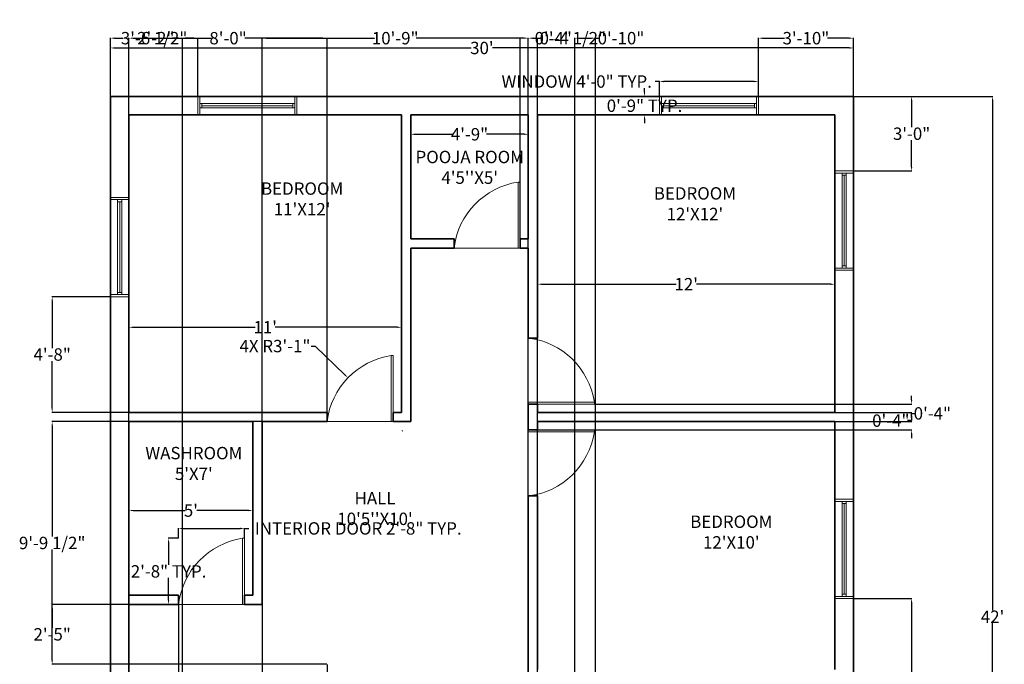
# Model space of a CAD drawing. Units: inches. Extents: x 897 to 1376, y 177 to 785.
# Tile 2 of 2: x 899 to 1376, y 473 to 785. Entities that reach past the tile are written whole.
import ezdxf

# ---------------------------------------------------------------- set-up
doc = ezdxf.new("R2010")
doc.units = ezdxf.units.IN
doc.header["$MEASUREMENT"] = 0
for name, color, linetype, lineweight in [('A-ANNO-DIMS', 2, 'Continuous', 13), ('A-AREA-IDEN', 7, 'Continuous', 18), ('A-DOOR', 3, 'Continuous', 18), ('A-GLAZ', 4, 'Continuous', 18), ('A-WALL', 7, 'Continuous', 35)]:
    doc.layers.add(name, color=color, linetype=linetype, lineweight=lineweight)
doc.styles.get("Standard").update_dxf_attribs({"font": 'arial.ttf'})
doc.dimstyles.get("Standard").update_dxf_attribs({"dimtxt": 6, "dimasz": 2, "dimexe": 0.18, "dimexo": 0.0625, "dimgap": 0.09, "dimtad": 0, "dimtih": 1, "dimtoh": 1, "dimdec": 0, "dimzin": 0, "dimdsep": 46, "dimlunit": 4, "dimtxsty": 'Standard', "dimcen": 0.09, "dimadec": 0, "dimazin": 0, "dimtfac": 1, "dimtdec": 0, "dimtofl": 0, "dimtmove": 0, "dimatfit": 3, "dimfxl": 1, "dimtolj": 1, "dimtzin": 0, "dimarcsym": 0})

# ---------------------------------------------------------------- blocks, each defined once
blk = doc.blocks.new('RFEGTHYUJU')
for p, q in [((1141.26, 706.37), (1140.26, 706.37)), ((1140.26, 706.37), (1140.26, 674.37)), ((1141.26, 674.37), (1141.26, 706.37)), ((1141.26, 674.37), (1109.26, 674.37))]:
    blk.add_line(p, q)
blk.add_arc((1145.82, 669.96), 36.83, 98.6921, 173.1267)
blk = doc.blocks.new('*D2')
at = {"layer": 'A-ANNO-DIMS', "color": 0, "lineweight": -2, "transparency": 16777216}
for p, q in [((951.76, 594.93), (951.76, 636.26)), ((953.76, 636.08), (1012.86, 636.08)), ((1081.76, 636.08), (1022.66, 636.08)), ((1083.76, 594.93), (1083.76, 636.26))]:
    blk.add_line(p, q, dxfattribs=at)
at = {"layer": 'A-ANNO-DIMS', "color": 0, "transparency": 16777216}
for points in [[(953.76, 636.41), (953.76, 635.74), (951.76, 636.08)], [(1081.76, 636.41), (1081.76, 635.74), (1083.76, 636.08)]]:
    blk.add_solid(points, dxfattribs=at)
at = {"layer": 'Defpoints', "color": 0, "transparency": 16777216}
for p in [(1083.76, 636.08), (951.76, 594.87), (1083.76, 594.87)]:
    blk.add_point(p, dxfattribs=at)
at = {"layer": 'A-ANNO-DIMS', "color": 0, "transparency": 16777216, "insert": (1017.76, 636.08), "char_height": 6, "attachment_point": 5}
blk.add_mtext("\\A1;11'", dxfattribs=at)
blk = doc.blocks.new('*D3')
at = {"layer": 'A-ANNO-DIMS', "color": 0, "lineweight": -2, "transparency": 16777216}
for p, q in [((1149.76, 594.93), (1149.76, 657.1)), ((1151.76, 656.92), (1216.86, 656.92)), ((1291.76, 656.92), (1226.66, 656.92)), ((1293.76, 594.93), (1293.76, 657.1))]:
    blk.add_line(p, q, dxfattribs=at)
at = {"layer": 'A-ANNO-DIMS', "color": 0, "transparency": 16777216}
for points in [[(1151.76, 657.25), (1151.76, 656.58), (1149.76, 656.92)], [(1291.76, 657.25), (1291.76, 656.58), (1293.76, 656.92)]]:
    blk.add_solid(points, dxfattribs=at)
at = {"layer": 'Defpoints', "color": 0, "transparency": 16777216}
for p in [(1293.76, 656.92), (1149.76, 594.87), (1293.76, 594.87)]:
    blk.add_point(p, dxfattribs=at)
at = {"layer": 'A-ANNO-DIMS', "color": 0, "transparency": 16777216, "insert": (1221.76, 656.92), "char_height": 6, "attachment_point": 5}
blk.add_mtext("\\A1;12'", dxfattribs=at)
blk = doc.blocks.new('*D4')
at = {"layer": 'A-ANNO-DIMS', "color": 0, "lineweight": -2, "transparency": 16777216}
for p, q in [((951.76, 590.3), (951.76, 547.15)), ((1011.76, 590.3), (1011.76, 547.15)), ((953.76, 547.33), (978.91, 547.33)), ((1009.76, 547.33), (984.61, 547.33))]:
    blk.add_line(p, q, dxfattribs=at)
at = {"layer": 'A-ANNO-DIMS', "color": 0, "transparency": 16777216}
for points in [[(953.76, 547.66), (953.76, 547), (951.76, 547.33)], [(1009.76, 547.66), (1009.76, 547), (1011.76, 547.33)]]:
    blk.add_solid(points, dxfattribs=at)
at = {"layer": 'Defpoints', "color": 0, "transparency": 16777216}
for p in [(951.76, 590.37), (1011.76, 590.37), (1011.76, 547.33)]:
    blk.add_point(p, dxfattribs=at)
at = {"layer": 'A-ANNO-DIMS', "color": 0, "transparency": 16777216, "insert": (981.76, 547.33), "char_height": 6, "attachment_point": 5}
blk.add_mtext("\\A1;5'", dxfattribs=at)
blk = doc.blocks.new('*D5')
at = {"layer": 'A-ANNO-DIMS', "color": 0, "lineweight": -2, "transparency": 16777216}
for p, q in [((1088.26, 738.8), (1088.26, 729.36)), ((1145.26, 738.8), (1145.26, 729.36)), ((1090.26, 729.54), (1108.57, 729.54)), ((1143.26, 729.54), (1124.94, 729.54))]:
    blk.add_line(p, q, dxfattribs=at)
at = {"layer": 'A-ANNO-DIMS', "color": 0, "transparency": 16777216}
for points in [[(1090.26, 729.87), (1090.26, 729.2), (1088.26, 729.54)], [(1143.26, 729.87), (1143.26, 729.2), (1145.26, 729.54)]]:
    blk.add_solid(points, dxfattribs=at)
at = {"layer": 'Defpoints', "color": 0, "transparency": 16777216}
for p in [(1088.26, 738.87), (1145.26, 738.87), (1145.26, 729.54)]:
    blk.add_point(p, dxfattribs=at)
at = {"layer": 'A-ANNO-DIMS', "color": 0, "transparency": 16777216, "insert": (1116.76, 729.54), "char_height": 6, "attachment_point": 5}
blk.add_mtext('\\A1;4\'-9"', dxfattribs=at)
blk = doc.blocks.new('*D6')
at = {"layer": 'A-ANNO-DIMS', "color": 0, "lineweight": -2, "transparency": 16777216}
for p, q in [((1302.82, 747.87), (1370.38, 747.87)), ((1370.2, 745.87), (1370.2, 498.97)), ((1370.2, 245.87), (1370.2, 492.76)), ((1302.82, 243.87), (1370.38, 243.87))]:
    blk.add_line(p, q, dxfattribs=at)
at = {"layer": 'A-ANNO-DIMS', "color": 0, "transparency": 16777216}
for points in [[(1369.87, 745.87), (1370.53, 745.87), (1370.2, 747.87)], [(1369.87, 245.87), (1370.53, 245.87), (1370.2, 243.87)]]:
    blk.add_solid(points, dxfattribs=at)
at = {"layer": 'Defpoints', "color": 0, "transparency": 16777216}
for p in [(1302.76, 747.87), (1302.76, 243.87), (1370.2, 243.87)]:
    blk.add_point(p, dxfattribs=at)
at = {"layer": 'A-ANNO-DIMS', "color": 0, "transparency": 16777216, "insert": (1370.2, 495.87), "char_height": 6, "attachment_point": 5}
blk.add_mtext("\\A1;42'", dxfattribs=at)
blk = doc.blocks.new('*D7')
at = {"layer": 'A-ANNO-DIMS', "color": 0, "lineweight": -2, "transparency": 16777216}
for p, q in [((942.76, 747.93), (942.76, 771.51)), ((944.76, 771.33), (1117.58, 771.33)), ((1300.76, 771.33), (1127.94, 771.33)), ((1302.76, 747.93), (1302.76, 771.51))]:
    blk.add_line(p, q, dxfattribs=at)
at = {"layer": 'A-ANNO-DIMS', "color": 0, "transparency": 16777216}
for points in [[(944.76, 771.66), (944.76, 770.99), (942.76, 771.33)], [(1300.76, 771.66), (1300.76, 770.99), (1302.76, 771.33)]]:
    blk.add_solid(points, dxfattribs=at)
at = {"layer": 'Defpoints', "color": 0, "transparency": 16777216}
for p in [(1302.76, 771.33), (942.76, 747.87), (1302.76, 747.87)]:
    blk.add_point(p, dxfattribs=at)
at = {"layer": 'A-ANNO-DIMS', "color": 0, "transparency": 16777216, "insert": (1122.76, 771.33), "char_height": 6, "attachment_point": 5}
blk.add_mtext("\\A1;30'", dxfattribs=at)
blk = doc.blocks.new('WIN-48IN-FRAMED')
for p, q in [((-24, 4.5), (-24, -4.5)), ((-23, 4.5), (-23, -4.5)), ((-23, 1), (23, 1)), ((-22, 1), (-22, -1)), ((22, 1), (22, -1)), ((23, 4.5), (23, -4.5)), ((24, 4.5), (24, -4.5)), ((-23, -1), (23, -1)), ((-22, 0), (22, 0))]:
    blk.add_line(p, q)
blk = doc.blocks.new('*D10')
at = {"layer": 'A-ANNO-DIMS', "color": 0, "lineweight": -2, "transparency": 16777216}
for p, q in [((975.76, 533.93), (975.76, 538.85)), ((977.76, 538.67), (1005.76, 538.67)), ((1007.76, 533.93), (1007.76, 538.85)), ((1007.76, 538.67), (1009.76, 538.67))]:
    blk.add_line(p, q, dxfattribs=at)
at = {"layer": 'A-ANNO-DIMS', "color": 0, "transparency": 16777216}
for points in [[(977.76, 539), (977.76, 538.33), (975.76, 538.67)], [(1005.76, 539), (1005.76, 538.33), (1007.76, 538.67)]]:
    blk.add_solid(points, dxfattribs=at)
at = {"layer": 'Defpoints', "color": 0, "transparency": 16777216}
for p in [(1007.76, 538.67), (975.76, 533.87), (1007.76, 533.87)]:
    blk.add_point(p, dxfattribs=at)
at = {"layer": 'A-ANNO-DIMS', "color": 0, "transparency": 16777216, "insert": (1062.84, 538.67), "char_height": 6, "attachment_point": 5}
blk.add_mtext('\\A1;INTERIOR DOOR 2\'-8" TYP.', dxfattribs=at)
blk = doc.blocks.new('*D11')
at = {"layer": 'A-ANNO-DIMS', "color": 0, "lineweight": -2, "transparency": 16777216}
for p, q in [((975.7, 533.87), (970.78, 533.87)), ((970.96, 531.87), (970.96, 521.02)), ((970.96, 503.87), (970.96, 514.71)), ((975.7, 501.87), (970.78, 501.87))]:
    blk.add_line(p, q, dxfattribs=at)
at = {"layer": 'A-ANNO-DIMS', "color": 0, "transparency": 16777216}
for points in [[(970.63, 531.87), (971.29, 531.87), (970.96, 533.87)], [(970.63, 503.87), (971.29, 503.87), (970.96, 501.87)]]:
    blk.add_solid(points, dxfattribs=at)
at = {"layer": 'Defpoints', "color": 0, "transparency": 16777216}
for p in [(970.96, 533.87), (975.76, 533.87), (975.76, 501.87)]:
    blk.add_point(p, dxfattribs=at)
at = {"layer": 'A-ANNO-DIMS', "color": 0, "transparency": 16777216, "insert": (970.96, 517.87), "char_height": 6, "attachment_point": 5}
blk.add_mtext('\\A1;2\'-8" TYP.', dxfattribs=at)
blk = doc.blocks.new('*D12')
at = {"layer": 'A-ANNO-DIMS', "color": 0, "lineweight": -2, "transparency": 16777216}
for p, q in [((1208.76, 755.07), (1206.76, 755.07)), ((1208.76, 747.93), (1208.76, 755.25)), ((1254.76, 755.07), (1210.76, 755.07)), ((1256.76, 747.93), (1256.76, 755.25))]:
    blk.add_line(p, q, dxfattribs=at)
at = {"layer": 'A-ANNO-DIMS', "color": 0, "transparency": 16777216}
for points in [[(1210.76, 755.4), (1210.76, 754.73), (1208.76, 755.07)], [(1254.76, 755.4), (1254.76, 754.73), (1256.76, 755.07)]]:
    blk.add_solid(points, dxfattribs=at)
at = {"layer": 'Defpoints', "color": 0, "transparency": 16777216}
for p in [(1208.76, 755.07), (1208.76, 747.87), (1256.76, 747.87)]:
    blk.add_point(p, dxfattribs=at)
at = {"layer": 'A-ANNO-DIMS', "color": 0, "transparency": 16777216, "insert": (1168.71, 755.07), "char_height": 6, "attachment_point": 5}
blk.add_mtext('\\A1;WINDOW 4\'-0" TYP.', dxfattribs=at)
blk = doc.blocks.new('*D13')
at = {"layer": 'A-ANNO-DIMS', "color": 0, "lineweight": -2, "transparency": 16777216}
for p, q in [((1201.56, 749.87), (1201.56, 751.87)), ((1208.7, 747.87), (1201.38, 747.87)), ((1208.7, 738.87), (1201.38, 738.87)), ((1201.56, 736.87), (1201.56, 734.87))]:
    blk.add_line(p, q, dxfattribs=at)
at = {"layer": 'A-ANNO-DIMS', "color": 0, "transparency": 16777216}
for points in [[(1201.23, 749.87), (1201.9, 749.87), (1201.56, 747.87)], [(1201.23, 736.87), (1201.9, 736.87), (1201.56, 738.87)]]:
    blk.add_solid(points, dxfattribs=at)
at = {"layer": 'Defpoints', "color": 0, "transparency": 16777216}
for p in [(1208.76, 747.87), (1201.56, 738.87), (1208.76, 738.87)]:
    blk.add_point(p, dxfattribs=at)
at = {"layer": 'A-ANNO-DIMS', "color": 0, "transparency": 16777216, "insert": (1201.56, 743.37), "char_height": 6, "attachment_point": 5}
blk.add_mtext('\\A1;0\'-9" TYP.', dxfattribs=at)
blk = doc.blocks.new('*D19')
at = {"layer": 'A-ANNO-DIMS', "color": 0, "lineweight": -2, "transparency": 16777216}
for p, q in [((942.76, 747.93), (942.76, 776.25)), ((944.76, 776.07), (948.88, 776.07)), ((983.12, 776.07), (978.99, 776.07)), ((985.12, 747.93), (985.12, 776.25))]:
    blk.add_line(p, q, dxfattribs=at)
at = {"layer": 'A-ANNO-DIMS', "color": 0, "transparency": 16777216}
for points in [[(944.76, 776.4), (944.76, 775.73), (942.76, 776.07)], [(983.12, 776.4), (983.12, 775.73), (985.12, 776.07)]]:
    blk.add_solid(points, dxfattribs=at)
at = {"layer": 'Defpoints', "color": 0, "transparency": 16777216}
for p in [(985.12, 776.07), (942.76, 747.87), (985.12, 747.87)]:
    blk.add_point(p, dxfattribs=at)
at = {"layer": 'A-ANNO-DIMS', "color": 0, "transparency": 16777216, "insert": (963.94, 776.07), "char_height": 6, "attachment_point": 5}
blk.add_mtext('\\A1;3\'-6 1/2"', dxfattribs=at)
blk = doc.blocks.new('*D20')
at = {"layer": 'A-ANNO-DIMS', "color": 0, "lineweight": -2, "transparency": 16777216}
for p, q in [((1256.76, 747.93), (1256.76, 776.25)), ((1258.76, 776.07), (1269.37, 776.07)), ((1300.76, 776.07), (1290.16, 776.07)), ((1302.76, 747.93), (1302.76, 776.25))]:
    blk.add_line(p, q, dxfattribs=at)
at = {"layer": 'A-ANNO-DIMS', "color": 0, "transparency": 16777216}
for points in [[(1258.76, 776.4), (1258.76, 775.73), (1256.76, 776.07)], [(1300.76, 776.4), (1300.76, 775.73), (1302.76, 776.07)]]:
    blk.add_solid(points, dxfattribs=at)
at = {"layer": 'Defpoints', "color": 0, "transparency": 16777216}
for p in [(1302.76, 776.07), (1256.76, 747.87), (1302.76, 747.87)]:
    blk.add_point(p, dxfattribs=at)
at = {"layer": 'A-ANNO-DIMS', "color": 0, "transparency": 16777216, "insert": (1279.76, 776.07), "char_height": 6, "attachment_point": 5}
blk.add_mtext('\\A1;3\'-10"', dxfattribs=at)
blk = doc.blocks.new('*D21')
at = {"layer": 'A-ANNO-DIMS', "color": 0, "lineweight": -2, "transparency": 16777216}
for p, q in [((942.7, 650.89), (914.38, 650.89)), ((914.56, 648.89), (914.56, 626.03)), ((914.56, 596.87), (914.56, 619.73)), ((951.7, 594.87), (914.38, 594.87))]:
    blk.add_line(p, q, dxfattribs=at)
at = {"layer": 'A-ANNO-DIMS', "color": 0, "transparency": 16777216}
for points in [[(914.23, 648.89), (914.89, 648.89), (914.56, 650.89)], [(914.23, 596.87), (914.89, 596.87), (914.56, 594.87)]]:
    blk.add_solid(points, dxfattribs=at)
at = {"layer": 'Defpoints', "color": 0, "transparency": 16777216}
for p in [(914.56, 650.89), (942.76, 650.89), (951.76, 594.87)]:
    blk.add_point(p, dxfattribs=at)
at = {"layer": 'A-ANNO-DIMS', "color": 0, "transparency": 16777216, "insert": (914.56, 622.88), "char_height": 6, "attachment_point": 5}
blk.add_mtext('\\A1;4\'-8"', dxfattribs=at)
blk = doc.blocks.new('*D23')
at = {"layer": 'A-ANNO-DIMS', "color": 0, "lineweight": -2, "transparency": 16777216}
for p, q in [((1302.82, 747.87), (1331.14, 747.87)), ((1330.96, 745.87), (1330.96, 732.97)), ((1330.96, 713.75), (1330.96, 726.65)), ((1302.82, 711.75), (1331.14, 711.75))]:
    blk.add_line(p, q, dxfattribs=at)
at = {"layer": 'A-ANNO-DIMS', "color": 0, "transparency": 16777216}
for points in [[(1330.63, 745.87), (1331.29, 745.87), (1330.96, 747.87)], [(1330.63, 713.75), (1331.29, 713.75), (1330.96, 711.75)]]:
    blk.add_solid(points, dxfattribs=at)
at = {"layer": 'Defpoints', "color": 0, "transparency": 16777216}
for p in [(1302.76, 747.87), (1302.76, 711.75), (1330.96, 711.75)]:
    blk.add_point(p, dxfattribs=at)
at = {"layer": 'A-ANNO-DIMS', "color": 0, "transparency": 16777216, "insert": (1330.96, 729.81), "char_height": 6, "attachment_point": 5}
blk.add_mtext('\\A1;3\'-0"', dxfattribs=at)
blk = doc.blocks.new('*D24')
at = {"layer": 'A-ANNO-DIMS', "color": 0, "lineweight": -2, "transparency": 16777216}
for p, q in [((1302.82, 504.76), (1331.14, 504.76)), ((1330.96, 502.76), (1330.96, 377.47)), ((1330.96, 245.87), (1330.96, 371.16)), ((1302.82, 243.87), (1331.14, 243.87))]:
    blk.add_line(p, q, dxfattribs=at)
at = {"layer": 'A-ANNO-DIMS', "color": 0, "transparency": 16777216}
for points in [[(1330.63, 502.76), (1331.29, 502.76), (1330.96, 504.76)], [(1330.63, 245.87), (1331.29, 245.87), (1330.96, 243.87)]]:
    blk.add_solid(points, dxfattribs=at)
at = {"layer": 'Defpoints', "color": 0, "transparency": 16777216}
for p in [(1302.76, 504.76), (1330.96, 504.76), (1302.76, 243.87)]:
    blk.add_point(p, dxfattribs=at)
at = {"layer": 'A-ANNO-DIMS', "color": 0, "transparency": 16777216, "insert": (1330.96, 374.32), "char_height": 6, "attachment_point": 5}
blk.add_mtext('\\A1;21\'-9"', dxfattribs=at)
blk = doc.blocks.new('*D29')
at = {"layer": 'A-ANNO-DIMS', "color": 0, "lineweight": -2, "transparency": 16777216}
for p, q in [((1145.26, 252.93), (1145.26, 776.25)), ((1147.26, 776.07), (1147.76, 776.07)), ((1149.76, 252.93), (1149.76, 776.25)), ((1149.76, 776.07), (1151.76, 776.07))]:
    blk.add_line(p, q, dxfattribs=at)
at = {"layer": 'A-ANNO-DIMS', "color": 0, "transparency": 16777216}
for points in [[(1147.26, 776.4), (1147.26, 775.73), (1145.26, 776.07)], [(1147.76, 776.4), (1147.76, 775.73), (1149.76, 776.07)]]:
    blk.add_solid(points, dxfattribs=at)
at = {"layer": 'Defpoints', "color": 0, "transparency": 16777216}
for p in [(1149.76, 776.07), (1145.26, 252.87), (1149.76, 252.87)]:
    blk.add_point(p, dxfattribs=at)
at = {"layer": 'A-ANNO-DIMS', "color": 0, "transparency": 16777216, "insert": (1166.81, 776.07), "char_height": 6, "attachment_point": 5}
blk.add_mtext('\\A1;0\'-4 1/2"', dxfattribs=at)
blk = doc.blocks.new('*D30')
at = {"layer": 'A-ANNO-DIMS', "color": 0, "lineweight": -2, "transparency": 16777216}
for p, q in [((951.76, 468.43), (951.76, 776.25)), ((953.76, 776.07), (956.64, 776.07)), ((975.76, 776.07), (972.87, 776.07)), ((977.76, 410.43), (977.76, 776.25))]:
    blk.add_line(p, q, dxfattribs=at)
at = {"layer": 'A-ANNO-DIMS', "color": 0, "transparency": 16777216}
for points in [[(953.76, 776.4), (953.76, 775.73), (951.76, 776.07)], [(975.76, 776.4), (975.76, 775.73), (977.76, 776.07)]]:
    blk.add_solid(points, dxfattribs=at)
at = {"layer": 'Defpoints', "color": 0, "transparency": 16777216}
for p in [(977.76, 776.07), (951.76, 468.37), (977.76, 410.37)]:
    blk.add_point(p, dxfattribs=at)
at = {"layer": 'A-ANNO-DIMS', "color": 0, "transparency": 16777216, "insert": (964.76, 776.07), "char_height": 6, "attachment_point": 5}
blk.add_mtext('\\A1;2\'-2"', dxfattribs=at)
blk = doc.blocks.new('*D32')
at = {"layer": 'A-ANNO-DIMS', "color": 0, "lineweight": -2, "transparency": 16777216}
for p, q in [((1167.76, 465.93), (1167.76, 776.25)), ((1169.76, 776.07), (1175.76, 776.07)), ((1177.76, 465.93), (1177.76, 776.25)), ((1177.76, 776.07), (1179.76, 776.07))]:
    blk.add_line(p, q, dxfattribs=at)
at = {"layer": 'A-ANNO-DIMS', "color": 0, "transparency": 16777216}
for points in [[(1169.76, 776.4), (1169.76, 775.73), (1167.76, 776.07)], [(1175.76, 776.4), (1175.76, 775.73), (1177.76, 776.07)]]:
    blk.add_solid(points, dxfattribs=at)
at = {"layer": 'Defpoints', "color": 0, "transparency": 16777216}
for p in [(1177.76, 776.07), (1167.76, 465.87), (1177.76, 465.87)]:
    blk.add_point(p, dxfattribs=at)
at = {"layer": 'A-ANNO-DIMS', "color": 0, "transparency": 16777216, "insert": (1190.15, 776.07), "char_height": 6, "attachment_point": 5}
blk.add_mtext('\\A1;0\'-10"', dxfattribs=at)
blk = doc.blocks.new('*D34')
at = {"layer": 'A-ANNO-DIMS', "color": 0, "lineweight": -2, "transparency": 16777216}
for p, q in [((951.76, 506.3), (951.76, 185.49)), ((975.76, 506.3), (975.76, 185.49)), ((953.76, 185.67), (955.64, 185.67)), ((973.76, 185.67), (971.87, 185.67))]:
    blk.add_line(p, q, dxfattribs=at)
at = {"layer": 'A-ANNO-DIMS', "color": 0, "transparency": 16777216}
for points in [[(953.76, 186), (953.76, 185.33), (951.76, 185.67)], [(973.76, 186), (973.76, 185.33), (975.76, 185.67)]]:
    blk.add_solid(points, dxfattribs=at)
at = {"layer": 'Defpoints', "color": 0, "transparency": 16777216}
for p in [(951.76, 506.37), (975.76, 506.37), (975.76, 185.67)]:
    blk.add_point(p, dxfattribs=at)
at = {"layer": 'A-ANNO-DIMS', "color": 0, "transparency": 16777216, "insert": (963.76, 185.67), "char_height": 6, "attachment_point": 5}
blk.add_mtext('\\A1;2\'-0"', dxfattribs=at)
blk = doc.blocks.new('*D36')
at = {"layer": 'A-ANNO-DIMS', "color": 0, "lineweight": -2, "transparency": 16777216}
for p, q in [((1016.26, 590.43), (1016.26, 776.25)), ((1018.26, 776.07), (1070.65, 776.07)), ((1143.26, 776.07), (1090.87, 776.07)), ((1145.26, 586.43), (1145.26, 776.25))]:
    blk.add_line(p, q, dxfattribs=at)
at = {"layer": 'A-ANNO-DIMS', "color": 0, "transparency": 16777216}
for points in [[(1018.26, 776.4), (1018.26, 775.73), (1016.26, 776.07)], [(1143.26, 776.4), (1143.26, 775.73), (1145.26, 776.07)]]:
    blk.add_solid(points, dxfattribs=at)
at = {"layer": 'Defpoints', "color": 0, "transparency": 16777216}
for p in [(1145.26, 776.07), (1016.26, 590.37), (1145.26, 586.37)]:
    blk.add_point(p, dxfattribs=at)
at = {"layer": 'A-ANNO-DIMS', "color": 0, "transparency": 16777216, "insert": (1080.76, 776.07), "char_height": 6, "attachment_point": 5}
blk.add_mtext('\\A1;10\'-9"', dxfattribs=at)
blk = doc.blocks.new('*D37')
at = {"layer": 'A-ANNO-DIMS', "color": 0, "lineweight": -2, "transparency": 16777216}
for p, q in [((1047.7, 590.37), (914.38, 590.37)), ((914.56, 588.37), (914.56, 534.81)), ((914.56, 474.87), (914.56, 528.42)), ((1047.7, 472.87), (914.38, 472.87))]:
    blk.add_line(p, q, dxfattribs=at)
at = {"layer": 'A-ANNO-DIMS', "color": 0, "transparency": 16777216}
for points in [[(914.23, 588.37), (914.89, 588.37), (914.56, 590.37)], [(914.23, 474.87), (914.89, 474.87), (914.56, 472.87)]]:
    blk.add_solid(points, dxfattribs=at)
at = {"layer": 'Defpoints', "color": 0, "transparency": 16777216}
for p in [(914.56, 590.37), (1047.76, 590.37), (1047.76, 472.87)]:
    blk.add_point(p, dxfattribs=at)
at = {"layer": 'A-ANNO-DIMS', "color": 0, "transparency": 16777216, "insert": (914.56, 531.62), "char_height": 6, "attachment_point": 5}
blk.add_mtext('\\A1;9\'-9 1/2"', dxfattribs=at)
blk = doc.blocks.new('*D38')
at = {"layer": 'A-ANNO-DIMS', "color": 0, "lineweight": -2, "transparency": 16777216}
for p, q in [((951.7, 501.87), (914.38, 501.87)), ((914.56, 499.87), (914.56, 490.52)), ((914.56, 474.87), (914.56, 484.21)), ((951.7, 472.87), (914.38, 472.87))]:
    blk.add_line(p, q, dxfattribs=at)
at = {"layer": 'A-ANNO-DIMS', "color": 0, "transparency": 16777216}
for points in [[(914.23, 499.87), (914.89, 499.87), (914.56, 501.87)], [(914.23, 474.87), (914.89, 474.87), (914.56, 472.87)]]:
    blk.add_solid(points, dxfattribs=at)
at = {"layer": 'Defpoints', "color": 0, "transparency": 16777216}
for p in [(914.56, 501.87), (951.76, 501.87), (951.76, 472.87)]:
    blk.add_point(p, dxfattribs=at)
at = {"layer": 'A-ANNO-DIMS', "color": 0, "transparency": 16777216, "insert": (914.56, 487.37), "char_height": 6, "attachment_point": 5}
blk.add_mtext('\\A1;2\'-5"', dxfattribs=at)
blk = doc.blocks.new('*D40')
at = {"layer": 'A-ANNO-DIMS', "color": 0, "lineweight": -2, "transparency": 16777216}
for p, q in [((1016.26, 501.8), (1016.26, 185.49)), ((1047.76, 472.8), (1047.76, 185.49)), ((1014.26, 185.67), (1012.26, 185.67)), ((1049.76, 185.67), (1051.76, 185.67))]:
    blk.add_line(p, q, dxfattribs=at)
at = {"layer": 'A-ANNO-DIMS', "color": 0, "transparency": 16777216}
for points in [[(1014.26, 186), (1014.26, 185.33), (1016.26, 185.67)], [(1049.76, 186), (1049.76, 185.33), (1047.76, 185.67)]]:
    blk.add_solid(points, dxfattribs=at)
at = {"layer": 'Defpoints', "color": 0, "transparency": 16777216}
for p in [(1016.26, 501.87), (1047.76, 472.87), (1016.26, 185.67)]:
    blk.add_point(p, dxfattribs=at)
at = {"layer": 'A-ANNO-DIMS', "color": 0, "transparency": 16777216, "insert": (1032.01, 185.67), "char_height": 6, "attachment_point": 5}
blk.add_mtext('\\A1;2\'-7 1/2"', dxfattribs=at)
blk = doc.blocks.new('*D42')
at = {"layer": 'A-ANNO-DIMS', "color": 0, "lineweight": -2, "transparency": 16777216}
for p, q in [((951.76, 594.93), (951.76, 776.25)), ((953.76, 776.07), (991.69, 776.07)), ((1045.76, 776.07), (1007.83, 776.07)), ((1047.76, 594.93), (1047.76, 776.25))]:
    blk.add_line(p, q, dxfattribs=at)
at = {"layer": 'A-ANNO-DIMS', "color": 0, "transparency": 16777216}
for points in [[(953.76, 776.4), (953.76, 775.73), (951.76, 776.07)], [(1045.76, 776.4), (1045.76, 775.73), (1047.76, 776.07)]]:
    blk.add_solid(points, dxfattribs=at)
at = {"layer": 'Defpoints', "color": 0, "transparency": 16777216}
for p in [(1047.76, 776.07), (951.76, 594.87), (1047.76, 594.87)]:
    blk.add_point(p, dxfattribs=at)
at = {"layer": 'A-ANNO-DIMS', "color": 0, "transparency": 16777216, "insert": (999.76, 776.07), "char_height": 6, "attachment_point": 5}
blk.add_mtext('\\A1;8\'-0"', dxfattribs=at)
blk = doc.blocks.new('*D43')
at = {"layer": 'A-ANNO-DIMS', "color": 0, "lineweight": -2, "transparency": 16777216}
for p, q in [((1139.26, 776.07), (1137.26, 776.07)), ((1141.26, 678.93), (1141.26, 776.25)), ((1145.26, 678.93), (1145.26, 776.25)), ((1147.26, 776.07), (1149.26, 776.07))]:
    blk.add_line(p, q, dxfattribs=at)
at = {"layer": 'A-ANNO-DIMS', "color": 0, "transparency": 16777216}
for points in [[(1139.26, 776.4), (1139.26, 775.73), (1141.26, 776.07)], [(1147.26, 776.4), (1147.26, 775.73), (1145.26, 776.07)]]:
    blk.add_solid(points, dxfattribs=at)
at = {"layer": 'Defpoints', "color": 0, "transparency": 16777216}
for p in [(1145.26, 776.07), (1141.26, 678.87), (1145.26, 678.87)]:
    blk.add_point(p, dxfattribs=at)
at = {"layer": 'A-ANNO-DIMS', "color": 0, "transparency": 16777216, "insert": (1157.32, 776.07), "char_height": 6, "attachment_point": 5}
blk.add_mtext('\\A1;0\'-4"', dxfattribs=at)
blk = doc.blocks.new('*D44')
at = {"layer": 'A-ANNO-DIMS', "color": 0, "lineweight": -2, "transparency": 16777216}
for p, q in [((1330.96, 600.87), (1330.96, 602.87)), ((1177.32, 598.87), (1331.14, 598.87)), ((1149.82, 594.87), (1331.14, 594.87)), ((1330.96, 592.87), (1330.96, 590.87)), ((1330.96, 590.87), (1328.96, 590.87))]:
    blk.add_line(p, q, dxfattribs=at)
at = {"layer": 'A-ANNO-DIMS', "color": 0, "transparency": 16777216}
for points in [[(1330.63, 600.87), (1331.29, 600.87), (1330.96, 598.87)], [(1330.63, 592.87), (1331.29, 592.87), (1330.96, 594.87)]]:
    blk.add_solid(points, dxfattribs=at)
at = {"layer": 'Defpoints', "color": 0, "transparency": 16777216}
for p in [(1177.26, 598.87), (1149.76, 594.87), (1330.96, 594.87)]:
    blk.add_point(p, dxfattribs=at)
at = {"layer": 'A-ANNO-DIMS', "color": 0, "transparency": 16777216, "insert": (1320.89, 590.87), "char_height": 6, "attachment_point": 5}
blk.add_mtext('\\A1;0\'-4"', dxfattribs=at)
blk = doc.blocks.new('*D45')
at = {"layer": 'A-ANNO-DIMS', "color": 0, "lineweight": -2, "transparency": 16777216}
for p, q in [((1330.96, 592.37), (1330.96, 594.37)), ((1330.96, 594.37), (1332.96, 594.37)), ((1149.82, 590.37), (1331.14, 590.37)), ((1149.82, 586.37), (1331.14, 586.37)), ((1330.96, 584.37), (1330.96, 582.37))]:
    blk.add_line(p, q, dxfattribs=at)
at = {"layer": 'A-ANNO-DIMS', "color": 0, "transparency": 16777216}
for points in [[(1330.63, 592.37), (1331.29, 592.37), (1330.96, 590.37)], [(1330.63, 584.37), (1331.29, 584.37), (1330.96, 586.37)]]:
    blk.add_solid(points, dxfattribs=at)
at = {"layer": 'Defpoints', "color": 0, "transparency": 16777216}
for p in [(1149.76, 590.37), (1330.96, 590.37), (1149.76, 586.37)]:
    blk.add_point(p, dxfattribs=at)
at = {"layer": 'A-ANNO-DIMS', "color": 0, "transparency": 16777216, "insert": (1341.02, 594.37), "char_height": 6, "attachment_point": 5}
blk.add_mtext('\\A1;0\'-4"', dxfattribs=at)
blk = doc.blocks.new('*D46')
at = {"layer": 'A-ANNO-DIMS', "color": 0, "lineweight": -2, "transparency": 16777216}
for p, q in [((1040, 626.96), (1042, 626.96)), ((1042, 626.96), (1056.43, 612.98)), ((1084.23, 585.96), (1084.41, 585.96)), ((1084.32, 585.87), (1084.32, 586.05))]:
    blk.add_line(p, q, dxfattribs=at)
at = {"layer": 'A-ANNO-DIMS', "color": 0, "transparency": 16777216}
blk.add_solid([(1056.67, 613.22), (1056.2, 612.74), (1057.87, 611.58)], dxfattribs=at)
at = {"layer": 'Defpoints', "color": 0, "transparency": 16777216}
for p in [(1057.87, 611.58), (1084.32, 585.96)]:
    blk.add_point(p, dxfattribs=at)
at = {"layer": 'A-ANNO-DIMS', "color": 0, "transparency": 16777216, "insert": (1022.5, 626.96), "char_height": 6, "attachment_point": 5}
blk.add_mtext('\\A1;4X R3\'-1"', dxfattribs=at)

msp = doc.modelspace()

# ---------------------------------------------------------------- linework, layer by layer
at = {"layer": 'A-WALL'}
for p, q in [((942.76, 747.87), (1302.76, 747.87)), ((942.76, 243.87), (942.76, 747.87)), ((1302.76, 747.87), (1302.76, 243.87)), ((951.76, 738.87), (1083.76, 738.87)), ((951.76, 594.87), (951.76, 738.87)), ((1083.76, 594.87), (1083.76, 738.87)), ((1088.26, 738.87), (1145.26, 738.87)), ((1088.26, 678.87), (1088.26, 738.87)), ((1145.26, 738.87), (1145.26, 678.87)), ((1149.76, 738.87), (1149.76, 630.87)), ((1149.76, 738.87), (1293.76, 738.87)), ((1293.76, 738.87), (1293.76, 594.87)), ((1088.26, 678.87), (1109.26, 678.87)), ((1109.26, 678.87), (1109.26, 674.37)), ((1141.26, 678.87), (1141.26, 674.37)), ((1141.26, 678.87), (1145.26, 678.87)), ((1088.26, 590.37), (1088.26, 674.37)), ((1088.26, 674.37), (1109.26, 674.37)), ((1141.26, 674.37), (1145.26, 674.37)), ((1145.26, 674.37), (1145.26, 630.87)), ((1145.26, 630.87), (1149.76, 630.87)), ((1145.26, 598.87), (1149.76, 598.87)), ((1145.26, 598.87), (1145.26, 586.37)), ((1149.76, 598.87), (1149.76, 594.87)), ((951.76, 594.87), (1047.76, 594.87)), ((1047.76, 590.37), (1047.76, 594.87)), ((1079.76, 590.37), (1079.76, 594.87)), ((1079.76, 594.87), (1083.76, 594.87)), ((1149.76, 594.87), (1293.76, 594.87)), ((951.76, 590.37), (1011.76, 590.37)), ((951.76, 506.37), (951.76, 590.37)), ((1011.76, 506.37), (1011.76, 590.37)), ((1016.26, 501.87), (1016.26, 590.37)), ((1016.26, 590.37), (1047.76, 590.37)), ((1079.76, 590.37), (1088.26, 590.37)), ((1149.76, 590.37), (1293.76, 590.37)), ((1149.76, 590.37), (1149.76, 586.37)), ((1293.76, 590.37), (1293.76, 470.37)), ((1145.26, 586.37), (1149.76, 586.37)), ((1145.26, 554.37), (1149.76, 554.37)), ((1145.26, 554.37), (1145.26, 465.87)), ((1149.76, 554.37), (1149.76, 470.37)), ((951.76, 506.37), (975.76, 506.37)), ((975.76, 501.87), (975.76, 506.37)), ((1007.76, 501.87), (1007.76, 506.37)), ((1007.76, 506.37), (1011.76, 506.37)), ((951.76, 501.87), (975.76, 501.87)), ((951.76, 472.87), (951.76, 501.87)), ((1007.76, 501.87), (1016.26, 501.87))]:
    msp.add_line(p, q, dxfattribs=at)

# ---------------------------------------------------------------- block references
at = {"layer": 'A-DOOR'}
for p in [(0, 0), (-61.5, -84), (-133.5, -172.5)]:
    msp.add_blockref('RFEGTHYUJU', p, dxfattribs=at)
at = {"layer": 'A-DOOR', "rotation": 270}
msp.add_blockref('RFEGTHYUJU', (470.89, 1740.12), dxfattribs=at)
at = {"layer": 'A-DOOR', "xscale": -1, "rotation": 270}
msp.add_blockref('RFEGTHYUJU', (470.89, -554.89), dxfattribs=at)
at = {"layer": 'A-GLAZ'}
msp.add_blockref('WIN-48IN-FRAMED', (1009.12, 743.37), dxfattribs=at)
for p, rotation in [((1232.77, 743.37), 180), ((1298.26, 687.75), 270.0000000000001), ((947.26, 674.89), 269.9999999999996), ((1298.26, 528.76), 270.0000000000002)]:
    msp.add_blockref('WIN-48IN-FRAMED', p, dxfattribs=dict(at, rotation=rotation))

# ---------------------------------------------------------------- texts
at = {"layer": 'A-AREA-IDEN', "char_height": 6, "attachment_point": 1}
for s, width, insert in [("\\pxqc;POOJA ROOM^J4'5''X5'", 221.9375, (1005.89, 721.53)), ("\\pxqc;BEDROOM^J11'X12'", 238.5137, (916.4, 706.23)), ("\\pxqc;BEDROOM^J12'X12'", 206.2822, (1122.83, 703.91)), ("\\pxqc;WASHROOM^J5'X7'", 151.028, (907.67, 578.13)), ("\\pxqc;HALL^J10'5''X10'", 174.0506, (983.95, 556.3)), ("\\pxqc;BEDROOM^J12'X10'", 200.4698, (1143.37, 544.91))]:
    msp.add_mtext_dynamic_manual_height_columns(s, width=width, gutter_width=30, heights=[0], dxfattribs=dict(at, insert=insert))

# ---------------------------------------------------------------- dimensions: what is measured, and where the dimension line sits
at = {"layer": 'A-ANNO-DIMS'}
for base, p1, p2, override, picture, middle in [((985.12, 776.07), (942.76, 747.87), (985.12, 747.87), {"dimdec": 1, "dimlfac": 1, "dimrnd": 0, "dimzin": 1, "dimdsep": 46, "dimlunit": 4, "dimfrac": 2}, '*D19', (963.94, 776.07)), ((1149.76, 776.07), (1145.26, 252.87), (1149.76, 252.87), {"dimdec": 1, "dimlfac": 1, "dimrnd": 0, "dimzin": 1, "dimdsep": 46, "dimlunit": 4, "dimfrac": 2}, '*D29', (1166.81, 776.07)), ((977.76, 776.07), (951.76, 468.37), (977.76, 410.37), {"dimdec": 1, "dimlfac": 1, "dimrnd": 0, "dimzin": 1, "dimdsep": 46, "dimlunit": 4, "dimfrac": 2}, '*D30', (964.76, 776.07)), ((1047.76, 776.07), (951.76, 594.87), (1047.76, 594.87), {"dimdec": 1, "dimlfac": 1, "dimrnd": 0, "dimzin": 1, "dimdsep": 46, "dimlunit": 4, "dimfrac": 2}, '*D42', (999.76, 776.07)), ((1145.26, 776.07), (1016.26, 590.37), (1145.26, 586.37), {"dimdec": 1, "dimlfac": 1, "dimrnd": 0, "dimzin": 1, "dimdsep": 46, "dimlunit": 4, "dimfrac": 2}, '*D36', (1080.76, 776.07)), ((1145.26, 776.07), (1141.26, 678.87), (1145.26, 678.87), {"dimdec": 1, "dimlfac": 1, "dimrnd": 0, "dimzin": 1, "dimdsep": 46, "dimlunit": 4, "dimfrac": 2}, '*D43', (1157.32, 776.07)), ((1177.76, 776.07), (1167.76, 465.87), (1177.76, 465.87), {"dimdec": 1, "dimlfac": 1, "dimrnd": 0, "dimzin": 1, "dimdsep": 46, "dimlunit": 4, "dimfrac": 2}, '*D32', (1190.15, 776.07)), ((1302.76, 776.07), (1256.76, 747.87), (1302.76, 747.87), {"dimdec": 1, "dimlfac": 1, "dimrnd": 0, "dimzin": 1, "dimdsep": 46, "dimlunit": 4, "dimfrac": 2}, '*D20', (1279.76, 776.07)), ((1302.76, 771.33), (942.76, 747.87), (1302.76, 747.87), {"dimclrd": 0, "dimclre": 0, "dimclrt": 0}, '*D7', (1122.76, 771.33)), ((1145.26, 729.54), (1088.26, 738.87), (1145.26, 738.87), {"dimclrd": 0, "dimclre": 0, "dimclrt": 0}, '*D5', (1116.76, 729.54)), ((1293.76, 656.92), (1149.76, 594.87), (1293.76, 594.87), {"dimclrd": 0, "dimclre": 0, "dimclrt": 0}, '*D3', (1221.76, 656.92)), ((1083.76, 636.08), (951.76, 594.87), (1083.76, 594.87), {"dimclrd": 0, "dimclre": 0, "dimclrt": 0}, '*D2', (1017.76, 636.08)), ((1011.76, 547.33), (951.76, 590.37), (1011.76, 590.37), {"dimclrd": 0, "dimclre": 0, "dimclrt": 0}, '*D4', (981.76, 547.33)), ((975.76, 185.67), (951.76, 506.37), (975.76, 506.37), {"dimdec": 1, "dimlfac": 1, "dimrnd": 0, "dimzin": 1, "dimdsep": 46, "dimlunit": 4, "dimfrac": 2}, '*D34', (963.76, 185.67)), ((1016.26, 185.67), (1047.76, 472.87), (1016.26, 501.87), {"dimdec": 1, "dimlfac": 1, "dimrnd": 0, "dimzin": 1, "dimdsep": 46, "dimlunit": 4, "dimfrac": 2}, '*D40', (1032.01, 185.67))]:
    dim = msp.add_linear_dim(base=base, p1=p1, p2=p2, dimstyle='Standard', override=override, dxfattribs=at)
    dim.commit()
    dim.dimension.update_dxf_attribs({"geometry": picture, "text_midpoint": middle})
for base, p1, p2, angle, text, picture, middle in [((1208.76, 755.07), (1256.76, 747.87), (1208.76, 747.87), 180, 'WINDOW <> TYP.', '*D12', (1168.71, 755.07)), ((1201.56, 738.87), (1208.76, 747.87), (1208.76, 738.87), 270, '<> TYP.', '*D13', (1201.56, 743.37)), ((970.96, 533.87), (975.76, 501.87), (975.76, 533.87), 90, '<> TYP.', '*D11', (970.96, 517.87))]:
    dim = msp.add_linear_dim(base=base, p1=p1, p2=p2, angle=angle, text=text, dimstyle='Standard', override={"dimdec": 1, "dimlfac": 1, "dimrnd": 0, "dimzin": 1, "dimdsep": 46, "dimlunit": 4, "dimfrac": 2}, dxfattribs=at)
    dim.commit()
    dim.dimension.update_dxf_attribs({"geometry": picture, "text_midpoint": middle})
for base, p1, p2, override, picture, middle in [((1370.2, 243.87), (1302.76, 747.87), (1302.76, 243.87), {"dimclrd": 0, "dimclre": 0, "dimclrt": 0}, '*D6', (1370.2, 495.87)), ((1330.96, 711.75), (1302.76, 747.87), (1302.76, 711.75), {"dimdec": 1, "dimlfac": 1, "dimrnd": 0, "dimzin": 1, "dimdsep": 46, "dimlunit": 4, "dimfrac": 2}, '*D23', (1330.96, 729.81)), ((914.56, 650.89), (951.76, 594.87), (942.76, 650.89), {"dimdec": 1, "dimlfac": 1, "dimrnd": 0, "dimzin": 1, "dimdsep": 46, "dimlunit": 4, "dimfrac": 2}, '*D21', (914.56, 622.88)), ((1330.96, 594.87), (1177.26, 598.87), (1149.76, 594.87), {"dimdec": 1, "dimlfac": 1, "dimrnd": 0, "dimzin": 1, "dimdsep": 46, "dimlunit": 4, "dimfrac": 2}, '*D44', (1320.89, 590.87)), ((1330.96, 590.37), (1149.76, 586.37), (1149.76, 590.37), {"dimdec": 1, "dimlfac": 1, "dimrnd": 0, "dimzin": 1, "dimdsep": 46, "dimlunit": 4, "dimfrac": 2}, '*D45', (1341.02, 594.37)), ((914.56, 590.37), (1047.76, 472.87), (1047.76, 590.37), {"dimdec": 1, "dimlfac": 1, "dimrnd": 0, "dimzin": 1, "dimdsep": 46, "dimlunit": 4, "dimfrac": 2}, '*D37', (914.56, 531.62)), ((914.56, 501.87), (951.76, 472.87), (951.76, 501.87), {"dimdec": 1, "dimlfac": 1, "dimrnd": 0, "dimzin": 1, "dimdsep": 46, "dimlunit": 4, "dimfrac": 2}, '*D38', (914.56, 487.37)), ((1330.96, 504.76), (1302.76, 243.87), (1302.76, 504.76), {"dimdec": 1, "dimlfac": 1, "dimrnd": 0, "dimzin": 1, "dimdsep": 46, "dimlunit": 4, "dimfrac": 2}, '*D24', (1330.96, 374.32))]:
    dim = msp.add_linear_dim(base=base, p1=p1, p2=p2, angle=90, dimstyle='Standard', override=override, dxfattribs=at)
    dim.commit()
    dim.dimension.update_dxf_attribs({"geometry": picture, "text_midpoint": middle})
dim = msp.add_radius_dim(center=(1084.32, 585.96), mpoint=(1057.87, 611.58), text='4X <>', dimstyle='Standard', override={"dimdec": 1, "dimlfac": 1, "dimrnd": 0, "dimzin": 1, "dimdsep": 46, "dimlunit": 4, "dimfrac": 2}, dxfattribs=at)
dim.commit()
dim.dimension.update_dxf_attribs({"geometry": '*D46', "text_midpoint": (1022.5, 626.96), "dimtype": 164})
dim = msp.add_linear_dim(base=(1007.76, 538.67), p1=(975.76, 533.87), p2=(1007.76, 533.87), text='INTERIOR DOOR <> TYP.', dimstyle='Standard', override={"dimdec": 1, "dimlfac": 1, "dimrnd": 0, "dimzin": 1, "dimdsep": 46, "dimlunit": 4, "dimfrac": 2}, dxfattribs=at)
dim.commit()
dim.dimension.update_dxf_attribs({"geometry": '*D10', "text_midpoint": (1062.84, 538.67)})

doc.saveas('drawing.dxf')
